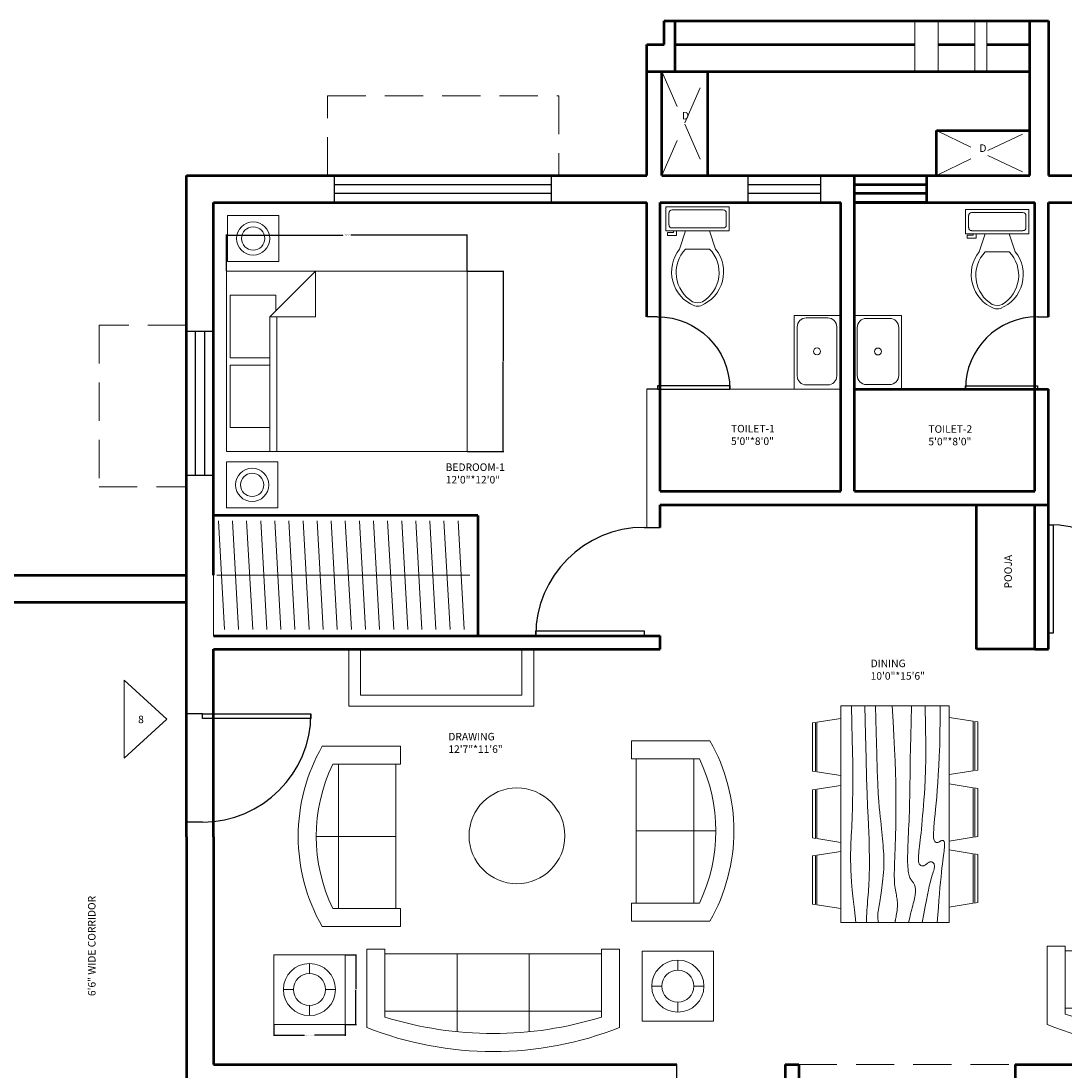
# Model space of a CAD drawing. Units: inches. Extents: x 4795 to 6024, y 2716 to 5025.
# Tile 18 of 19: x 5473 to 5820, y 4676 to 5025. Entities that reach past the tile are written whole.
import ezdxf

# ---------------------------------------------------------------- set-up
doc = ezdxf.new("R2010")
doc.units = ezdxf.units.IN
doc.linetypes.add('DASHED', pattern=[19.05, 12.7, -6.35])
for name, color, linetype, lineweight in [('A-ANNO-DIMS', 2, 'Continuous', 18), ('A-ANNO-TEXT', 7, 'Continuous', 18), ('A-AREA-IDEN', 3, 'Continuous', 18), ('A-DOOR', 4, 'Continuous', 25), ('A-FLOR-FIXT', 9, 'Continuous', 18), ('A-FURN', 8, 'Continuous', 18), ('A-GLAZ', 4, 'Continuous', 25), ('A-WALL', 7, 'Continuous', 50), ('A-WALL-OVHD', 8, 'DASHED', 18)]:
    doc.layers.add(name, color=color, linetype=linetype, lineweight=lineweight)
doc.styles.get("Standard").update_dxf_attribs({"font": 'arial.ttf'})
doc.dimstyles.get("Standard").update_dxf_attribs({"dimtxt": 0.18, "dimasz": 0.18, "dimexe": 0.18, "dimexo": 0.0625, "dimgap": 0.09, "dimtad": 0, "dimtih": 1, "dimtoh": 1, "dimdec": 4, "dimzin": 0, "dimdsep": 46, "dimtxsty": 'Standard', "dimcen": 0.09, "dimadec": 0, "dimazin": 0, "dimtfac": 1, "dimtdec": 4, "dimtofl": 0, "dimtmove": 0, "dimatfit": 3, "dimfxl": 1, "dimtolj": 1, "dimtzin": 0, "dimarcsym": 0})

# ---------------------------------------------------------------- blocks, each defined once
blk = doc.blocks.new('*U2')
for p, q in [((0, 0), (0, -6)), ((40, 0), (40, -6))]:
    blk.add_line(p, q)
blk.add_lwpolyline([(0, 0), (0, 40), (1.75, 40), (1.75, 0)], close=True)
blk.add_arc((0, 0), 40, 0, 90)
blk = doc.blocks.new('Bed - Queen')
for p, q in [((0, -80.00003), (0, 0)), ((0, 0), (59.99999, 0)), ((59.99999, 0), (59.99999, -80.00003)), ((7.99999, -1.2), (28.79998, -1.2)), ((7.99999, -14.4), (7.99999, -1.2)), ((28.79998, -1.2), (28.79998, -14.4)), ((31.19999, -1.2), (51.99999, -1.2)), ((31.19999, -14.4), (31.19999, -1.2)), ((51.99999, -1.2), (51.99999, -16.4)), ((0, -14.4), (44.8, -14.4)), ((44.8, -16.8), (0, -16.8)), ((59.99999, -29.6), (44.8, -14.4)), ((44.8, -14.4), (44.8, -29.6)), ((51.99999, -16.4), (46.79936, -16.4)), ((44.8, -29.6), (59.99999, -29.6)), ((59.99999, -80.00003), (0, -80.00003))]:
    blk.add_line(p, q)
blk = doc.blocks.new('Toilet - top')
for p, q in [((9.5, -6), (9.5, -2)), ((-10, -8.5), (-8, -8.5)), ((-10, -9.5), (-10, -8.5)), ((-7, -9.5), (-10, -9.5)), ((-8, -8.5), (-8, -8)), ((-7, -8), (-7, -9.5)), ((-4, -8), (-6, -14)), ((4, -8), (6, -14)), ((4, -14), (-4, -14))]:
    blk.add_line(p, q)
blk.add_lwpolyline([(10.5, -8), (10.5, 0), (-10.5, 0), (-10.5, -8)], close=True)
for points in [[(-9.5, -2), (-9.5, -6)], [(8.5, -1), (-8.5, -1)], [(-8.5, -7), (8.5, -7)]]:
    blk.add_lwpolyline(points)
for centre, radius, start, end in [((-8.62, -1.88), 0.884, 81.8699, 188.1301), ((8.62, -1.88), 0.884, 351.8699, 98.1301), ((-8.62, -6.12), 0.884, 171.8699, 278.1301), ((8.62, -6.12), 0.884, 261.8699, 8.1301), ((3.52, -21.58), 12.17, 141.4691, 247.9714), ((4.2, -21.82), 11.33, 136.3677, 238.9468), ((-3.52, -21.58), 12.17, 292.0284, 38.5307), ((-4.2, -21.82), 11.33, 301.053, 43.6321), ((0, -27.88), 4, 245.7318, 294.2682), ((0, -29), 4, 254.8605, 285.1395)]:
    blk.add_arc(centre, radius, start, end)
blk = doc.blocks.new('Sofa - Roundback 7 ft.')
for p, q in [((-12.00002, -32.4421), (-12.00003, -6.5971)), ((11.99997, -32.4421), (11.99998, -6.5971)), ((-36.000027, -34), (-36.000027, -11.4696)), ((-35.999844, -13.3819), (35.9998, -13.3819)), ((35.99998, -34), (35.99998, -11.4696)), ((-36.000027, -32.4421), (35.99998, -32.4421))]:
    blk.add_line(p, q)
for points in [[(-36.000027, -34), (-42.000027, -34), (-42.000027, -8)], [(41.99998, -8), (41.99998, -34), (35.99998, -34)]]:
    blk.add_lwpolyline(points)
for centre, radius, start, end in [((0, -114.25), 114.25, 68.43141, 111.5686), ((-0.00001, -127.1968), 121.1968, 72.72033, 107.2797)]:
    blk.add_arc(centre, radius, start, end)
blk = doc.blocks.new('Sofa - Roundback Loveseat 5 ft.')
for p, q in [((0, -32.44198), (0, -5.99998)), ((-24, -33.99998), (-24, -11.46958)), ((-23.9998, -13.38178), (23.99986, -13.38178)), ((24.00004, -33.99998), (24.00004, -11.46958)), ((-24, -32.44198), (24.00004, -32.44198))]:
    blk.add_line(p, q)
for points in [[(-24, -33.99998), (-30, -33.99998), (-30, -7.99998)], [(30.00004, -7.99998), (30.00004, -33.99998), (24.00004, -33.99998)]]:
    blk.add_lwpolyline(points)
for centre, radius, start, end in [((0, -60.24998), 60.24998, 60.13715, 119.8628), ((0, -61.38438), 55.38444, 64.32083, 115.6792)]:
    blk.add_arc(centre, radius, start, end)
blk = doc.blocks.new('WIN-48')
for p, q in [((0, 0), (0, 48)), ((0, 48), (9, 48)), ((3, 0), (3, 48)), ((6, 48), (6, 0)), ((9, 48), (9, 0)), ((9, 0), (0, 0))]:
    blk.add_line(p, q)
blk = doc.blocks.new('WIN-72')
for p, q in [((0, 0), (0, 9)), ((0, 9), (72, 9)), ((72, 9), (72, 0)), ((0, 6), (72, 6)), ((72, 3), (0, 3)), ((72, 0), (0, 0))]:
    blk.add_line(p, q)
blk = doc.blocks.new('WIN-24')
for p, q in [((0, 0), (0, 9)), ((0, 9), (24, 9)), ((24, 9), (24, 0)), ((0, 6), (24, 6)), ((24, 3), (0, 3)), ((24, 0), (0, 0))]:
    blk.add_line(p, q)
blk = doc.blocks.new('CHAIR-DINING')
for p, q in [((8, 17.72), (0, 18.97)), ((8, 17.71), (8, 1.25)), ((9.5, 17.48), (8.5, 17.64)), ((8.5, 1.33), (8.5, 17.64)), ((9.5, 17.48), (9.5, 1.48)), ((0, 0), (8, 1.25)), ((8.5, 1.33), (9.5, 1.48))]:
    blk.add_line(p, q)
blk = doc.blocks.new('LAMP-SIDE')
for p, q in [((11.88, 20.25), (11.88, 16.92)), ((3.23, 11.6), (6.56, 11.6)), ((17.2, 11.6), (20.54, 11.6)), ((11.88, 6.28), (11.88, 2.94))]:
    blk.add_line(p, q)
blk.add_lwpolyline([(23.76, 23.19), (0, 23.19), (0, 0), (23.76, 0)], close=True)
for radius in [8.66, 5.32]:
    blk.add_circle((11.88, 11.6), radius)
blk = doc.blocks.new('*D23')
at = {"layer": 'A-ANNO-DIMS', "color": 0, "lineweight": -2, "transparency": 16777216}
for p, q in [((5557.24, 4691.68), (5557.24, 4688)), ((5581, 4691.68), (5581, 4688)), ((5557.42, 4688.18), (5567.46, 4688.18)), ((5580.82, 4688.18), (5570.79, 4688.18))]:
    blk.add_line(p, q, dxfattribs=at)
at = {"layer": 'A-ANNO-DIMS', "color": 0, "lineweight": 100, "transparency": 16777216}
for points in [[(5557.42, 4688.21), (5557.42, 4688.15), (5557.24, 4688.18)], [(5580.82, 4688.21), (5580.82, 4688.15), (5581, 4688.18)]]:
    blk.add_solid(points, dxfattribs=at)
at = {"layer": 'DEFPOINTS', "color": 0, "lineweight": 100, "transparency": 16777216}
for p in [(5557.24, 4691.74), (5581, 4691.74), (5581, 4688.18)]:
    blk.add_point(p, dxfattribs=at)
at = {"layer": 'A-ANNO-DIMS', "color": 0, "transparency": 16777216, "insert": (5569.12, 4688.18), "char_height": 0.18, "attachment_point": 5}
blk.add_mtext('\\A1;SIDE TABLE LAMP 24 TYP.', dxfattribs=at)
blk = doc.blocks.new('*D24')
at = {"layer": 'A-ANNO-DIMS', "color": 0, "lineweight": -2, "transparency": 16777216}
for p, q in [((5581.07, 4714.94), (5584.75, 4714.94)), ((5584.57, 4714.76), (5584.57, 4703.52)), ((5584.57, 4691.92), (5584.57, 4703.16)), ((5581.07, 4691.74), (5584.75, 4691.74))]:
    blk.add_line(p, q, dxfattribs=at)
at = {"layer": 'A-ANNO-DIMS', "color": 0, "lineweight": 100, "transparency": 16777216}
for points in [[(5584.54, 4714.76), (5584.6, 4714.76), (5584.57, 4714.94)], [(5584.54, 4691.92), (5584.6, 4691.92), (5584.57, 4691.74)]]:
    blk.add_solid(points, dxfattribs=at)
at = {"layer": 'DEFPOINTS', "color": 0, "lineweight": 100, "transparency": 16777216}
for p in [(5581, 4714.94), (5584.57, 4714.94), (5581, 4691.74)]:
    blk.add_point(p, dxfattribs=at)
at = {"layer": 'A-ANNO-DIMS', "color": 0, "transparency": 16777216, "insert": (5584.57, 4703.34), "char_height": 0.18, "attachment_point": 5}
blk.add_mtext('\\A1;23 TYP.', dxfattribs=at)
blk = doc.blocks.new('*D25')
at = {"layer": 'A-ANNO-DIMS', "color": 0, "lineweight": -2, "transparency": 16777216}
for p, q in [((5541.53, 4942.23), (5541.53, 4954.35)), ((5541.71, 4954.17), (5580.22, 4954.17)), ((5621.35, 4954.17), (5582.83, 4954.17)), ((5621.53, 4942.23), (5621.53, 4954.35))]:
    blk.add_line(p, q, dxfattribs=at)
at = {"layer": 'A-ANNO-DIMS', "color": 0, "lineweight": 100, "transparency": 16777216}
for points in [[(5541.71, 4954.2), (5541.71, 4954.14), (5541.53, 4954.17)], [(5621.35, 4954.2), (5621.35, 4954.14), (5621.53, 4954.17)]]:
    blk.add_solid(points, dxfattribs=at)
at = {"layer": 'DEFPOINTS', "color": 0, "lineweight": 100, "transparency": 16777216}
for p in [(5541.53, 4954.17), (5541.53, 4942.17), (5621.53, 4942.17)]:
    blk.add_point(p, dxfattribs=at)
at = {"layer": 'A-ANNO-DIMS', "color": 0, "transparency": 16777216, "insert": (5581.53, 4954.17), "char_height": 0.18, "attachment_point": 5}
blk.add_mtext('\\A1;QUEEN BED 80 TYP.', dxfattribs=at)
blk = doc.blocks.new('*D26')
at = {"layer": 'A-ANNO-DIMS', "color": 0, "lineweight": -2, "transparency": 16777216}
for p, q in [((5621.59, 4942.17), (5633.71, 4942.17)), ((5633.53, 4941.99), (5633.53, 4912.35)), ((5633.53, 4882.35), (5633.53, 4911.99)), ((5621.59, 4882.17), (5633.71, 4882.17))]:
    blk.add_line(p, q, dxfattribs=at)
at = {"layer": 'A-ANNO-DIMS', "color": 0, "lineweight": 100, "transparency": 16777216}
for points in [[(5633.5, 4941.99), (5633.56, 4941.99), (5633.53, 4942.17)], [(5633.5, 4882.35), (5633.56, 4882.35), (5633.53, 4882.17)]]:
    blk.add_solid(points, dxfattribs=at)
at = {"layer": 'DEFPOINTS', "color": 0, "lineweight": 100, "transparency": 16777216}
for p in [(5621.53, 4942.17), (5633.53, 4942.17), (5621.53, 4882.17)]:
    blk.add_point(p, dxfattribs=at)
at = {"layer": 'A-ANNO-DIMS', "color": 0, "transparency": 16777216, "insert": (5633.53, 4912.17), "char_height": 0.18, "attachment_point": 5}
blk.add_mtext('\\A1;60 TYP.', dxfattribs=at)

msp = doc.modelspace()

# ---------------------------------------------------------------- linework, layer by layer
at = {"layer": 'A-FLOR-FIXT'}
for points in [[(5745.72, 4902.99), (5730.23, 4902.99), (5730.23, 4927.41), (5745.72, 4927.41)], [(5750.22, 4902.99), (5765.94, 4902.99), (5765.94, 4927.41), (5750.22, 4927.41)]]:
    msp.add_lwpolyline(points, close=True, dxfattribs=at)
for points in [[(5734.23, 4926.65), (5741.38, 4926.65, -0.414214), (5744.38, 4923.65), (5744.38, 4907.34, -0.414214), (5741.38, 4904.34), (5734.23, 4904.34, -0.414214), (5731.23, 4907.34), (5731.23, 4923.65, -0.414214)], [(5754.16, 4926.44), (5761.96, 4926.44, -0.414214), (5764.96, 4923.44), (5764.96, 4907.49, -0.414214), (5761.96, 4904.49), (5754.16, 4904.49, -0.414214), (5751.16, 4907.49), (5751.16, 4923.44, -0.414214)]]:
    msp.add_lwpolyline(points, format="xyb", close=True, dxfattribs=at)
for centre in [(5737.81, 4915.49), (5758.06, 4915.47)]:
    msp.add_circle(centre, 1.15, dxfattribs=at)
at = {"layer": 'A-FURN'}
for p, q in [((5681.22, 4902.99), (5745.72, 4902.99)), ((5681.22, 4856.98), (5681.22, 4902.99)), ((5538.87, 4859.18), (5540.89, 4823.01)), ((5543.56, 4859.18), (5545.57, 4823.01)), ((5548.24, 4859.18), (5550.26, 4823.01)), ((5552.93, 4859.18), (5554.95, 4823.01)), ((5557.61, 4859.18), (5559.63, 4823.01)), ((5562.3, 4859.18), (5564.32, 4823.01)), ((5566.98, 4859.18), (5569, 4823.01)), ((5571.67, 4859.18), (5573.69, 4823.01)), ((5576.36, 4859.18), (5578.37, 4823.01)), ((5581.04, 4859.18), (5583.06, 4823.01)), ((5585.73, 4859.18), (5587.75, 4823.01)), ((5590.41, 4859.18), (5592.43, 4823.01)), ((5595.1, 4859.18), (5597.12, 4823.01)), ((5599.78, 4859.18), (5601.8, 4823.01)), ((5604.47, 4859.18), (5606.49, 4823.01)), ((5609.16, 4859.18), (5611.17, 4823.01)), ((5613.84, 4859.18), (5615.86, 4823.01)), ((5618.53, 4859.18), (5620.55, 4823.01)), ((5537.22, 4820.98), (5537.22, 4841.09)), ((5538.32, 4841.1), (5622.4, 4841.1)), ((5582.22, 4816.48), (5582.22, 4797.51)), ((5586.13, 4816.48), (5586.13, 4801.2)), ((5639.68, 4801.2), (5639.68, 4816.48)), ((5643.75, 4797.51), (5643.75, 4816.48)), ((5507.59, 4806.23), (5507.59, 4780.26)), ((5521.76, 4793.24), (5507.59, 4806.23)), ((5586.13, 4801.2), (5639.68, 4801.2)), ((5582.22, 4797.51), (5643.75, 4797.51)), ((5745.76, 4797.66), (5745.76, 4725.66)), ((5781.76, 4797.66), (5745.76, 4797.66)), ((5781.76, 4725.66), (5781.76, 4797.66)), ((5507.59, 4780.26), (5521.76, 4793.24)), ((5745.76, 4725.66), (5781.76, 4725.66))]:
    msp.add_line(p, q, dxfattribs=at)
for points in [[(5770.32, 5025.34), (5778.07, 5025.34), (5778.07, 5008.52), (5770.32, 5008.52)], [(5790.29, 5025.34), (5794.24, 5025.34), (5794.24, 5008.52), (5790.29, 5008.52)], [(5541.86, 4960.71), (5558.98, 4960.71), (5558.98, 4945.37), (5541.86, 4945.37)], [(5541.53, 4878.78), (5558.65, 4878.78), (5558.65, 4863.44), (5541.53, 4863.44)]]:
    msp.add_lwpolyline(points, close=True, dxfattribs=at)
for points in [[(5749.26, 4797.66), (5749.43, 4791.75), (5749.55, 4786.69), (5749.64, 4782.39), (5749.69, 4778.74), (5749.72, 4775.63), (5749.72, 4772.96), (5749.71, 4770.63), (5749.68, 4768.53), (5749.65, 4766.58), (5749.6, 4764.75), (5749.56, 4763.03), (5749.5, 4761.41), (5749.45, 4759.89), (5749.39, 4758.46), (5749.33, 4757.11), (5749.26, 4755.83), (5749.2, 4754.6), (5749.14, 4753.42), (5749.09, 4752.27), (5749.04, 4751.11), (5749, 4749.94), (5748.98, 4748.73), (5748.97, 4747.46), (5748.97, 4746.12), (5749, 4744.67), (5749.06, 4743.04), (5749.16, 4741.18), (5749.32, 4739), (5749.55, 4736.43), (5749.86, 4733.4), (5750.26, 4729.83), (5750.76, 4725.66)], [(5753.76, 4797.66), (5753.95, 4788.06), (5754.13, 4780.13), (5754.31, 4773.64), (5754.48, 4768.4), (5754.64, 4764.18), (5754.78, 4760.78), (5754.91, 4757.98), (5755.01, 4755.58), (5755.1, 4753.38), (5755.16, 4751.36), (5755.2, 4749.49), (5755.22, 4747.76), (5755.23, 4746.17), (5755.22, 4744.7), (5755.21, 4743.34), (5755.18, 4742.08), (5755.15, 4740.9), (5755.1, 4739.79), (5755.05, 4738.74), (5755, 4737.73), (5754.94, 4736.75), (5754.87, 4735.78), (5754.8, 4734.81), (5754.72, 4733.83), (5754.64, 4732.81), (5754.56, 4731.78), (5754.49, 4730.73), (5754.41, 4729.68), (5754.35, 4728.64), (5754.31, 4727.61), (5754.27, 4726.62), (5754.26, 4725.66)], [(5757.26, 4797.66), (5757.45, 4788.84), (5757.64, 4781.74), (5757.82, 4776.13), (5758, 4771.77), (5758.18, 4768.43), (5758.35, 4765.9), (5758.52, 4763.92), (5758.68, 4762.28), (5758.83, 4760.79), (5758.98, 4759.39), (5759.11, 4758.07), (5759.24, 4756.83), (5759.36, 4755.65), (5759.48, 4754.53), (5759.58, 4753.45), (5759.68, 4752.41), (5759.77, 4751.39), (5759.85, 4750.39), (5759.92, 4749.39), (5759.97, 4748.41), (5760.01, 4747.42), (5760.03, 4746.43), (5760.03, 4745.43), (5760.01, 4744.41), (5759.97, 4743.37), (5759.91, 4742.31), (5759.83, 4741.26), (5759.73, 4740.21), (5759.63, 4739.18), (5759.51, 4738.19), (5759.39, 4737.23), (5759.26, 4736.33), (5759.14, 4735.48), (5759.01, 4734.69), (5758.89, 4733.94), (5758.77, 4733.24), (5758.65, 4732.56), (5758.53, 4731.9), (5758.42, 4731.26), (5758.31, 4730.62), (5758.2, 4729.98), (5758.11, 4729.33), (5758.03, 4728.69), (5757.99, 4728.06), (5757.98, 4727.44), (5758.02, 4726.83), (5758.11, 4726.23), (5758.26, 4725.66)], [(5762.76, 4797.66), (5763.1, 4792.45), (5763.38, 4787.68), (5763.6, 4783.31), (5763.77, 4779.32), (5763.89, 4775.66), (5763.98, 4772.31), (5764.03, 4769.24), (5764.06, 4766.41), (5764.06, 4763.79), (5764.05, 4761.37), (5764.03, 4759.13), (5763.99, 4757.04), (5763.94, 4755.11), (5763.89, 4753.3), (5763.83, 4751.6), (5763.76, 4749.99), (5763.7, 4748.47), (5763.64, 4747.02), (5763.59, 4745.66), (5763.55, 4744.38), (5763.51, 4743.18), (5763.49, 4742.06), (5763.49, 4741.02), (5763.51, 4740.08), (5763.56, 4739.21), (5763.62, 4738.42), (5763.7, 4737.7), (5763.78, 4737.04), (5763.88, 4736.44), (5763.98, 4735.87), (5764.08, 4735.33), (5764.18, 4734.83), (5764.27, 4734.33), (5764.35, 4733.85), (5764.42, 4733.37), (5764.47, 4732.89), (5764.51, 4732.4), (5764.53, 4731.9), (5764.53, 4731.37), (5764.51, 4730.83), (5764.47, 4730.25), (5764.41, 4729.66), (5764.34, 4729.07), (5764.25, 4728.5), (5764.17, 4727.96), (5764.08, 4727.47), (5764, 4727.04), (5763.93, 4726.7), (5763.88, 4726.45), (5763.83, 4726.27), (5763.8, 4726.16), (5763.78, 4726.07), (5763.77, 4726), (5763.77, 4725.92), (5763.76, 4725.81), (5763.76, 4725.66)], [(5769.26, 4797.66), (5769.1, 4792.37), (5768.97, 4787.73), (5768.88, 4783.65), (5768.82, 4780.09), (5768.77, 4776.96), (5768.74, 4774.21), (5768.71, 4771.77), (5768.68, 4769.58), (5768.65, 4767.57), (5768.6, 4765.72), (5768.56, 4764), (5768.5, 4762.4), (5768.45, 4760.89), (5768.39, 4759.44), (5768.33, 4758.04), (5768.26, 4756.66), (5768.2, 4755.29), (5768.14, 4753.92), (5768.09, 4752.59), (5768.03, 4751.28), (5767.99, 4750.03), (5767.96, 4748.83), (5767.94, 4747.7), (5767.93, 4746.66), (5767.94, 4745.71), (5767.96, 4744.84), (5768, 4744.06), (5768.06, 4743.36), (5768.13, 4742.73), (5768.21, 4742.17), (5768.31, 4741.68), (5768.43, 4741.24), (5768.56, 4740.86), (5768.71, 4740.53), (5768.86, 4740.23), (5769.02, 4739.97), (5769.19, 4739.73), (5769.36, 4739.51), (5769.52, 4739.29), (5769.68, 4739.08), (5769.83, 4738.85), (5769.97, 4738.62), (5770.11, 4738.37), (5770.22, 4738.11), (5770.32, 4737.82), (5770.41, 4737.52), (5770.47, 4737.19), (5770.51, 4736.83), (5770.53, 4736.44), (5770.53, 4736.02), (5770.51, 4735.57), (5770.46, 4735.11), (5770.4, 4734.62), (5770.31, 4734.12), (5770.21, 4733.6), (5770.1, 4733.08), (5769.96, 4732.53), (5769.81, 4731.95), (5769.63, 4731.29), (5769.43, 4730.52), (5769.2, 4729.61), (5768.93, 4728.52), (5768.62, 4727.21), (5768.26, 4725.66)], [(5773.76, 4797.66), (5773.91, 4790.64), (5773.97, 4784.83), (5773.96, 4780.08), (5773.9, 4776.23), (5773.79, 4773.1), (5773.66, 4770.54), (5773.51, 4768.37), (5773.35, 4766.45), (5773.19, 4764.63), (5773.05, 4762.88), (5772.91, 4761.22), (5772.77, 4759.63), (5772.64, 4758.13), (5772.52, 4756.72), (5772.39, 4755.39), (5772.26, 4754.16), (5772.14, 4753.02), (5772.02, 4751.97), (5771.9, 4751.01), (5771.8, 4750.13), (5771.7, 4749.33), (5771.62, 4748.62), (5771.56, 4747.98), (5771.51, 4747.41), (5771.49, 4746.91), (5771.5, 4746.48), (5771.52, 4746.11), (5771.57, 4745.78), (5771.63, 4745.51), (5771.71, 4745.28), (5771.81, 4745.08), (5771.93, 4744.91), (5772.06, 4744.76), (5772.21, 4744.64), (5772.37, 4744.55), (5772.53, 4744.48), (5772.71, 4744.44), (5772.89, 4744.43), (5773.08, 4744.45), (5773.26, 4744.49), (5773.45, 4744.57), (5773.64, 4744.67), (5773.83, 4744.79), (5774.01, 4744.93), (5774.2, 4745.07), (5774.39, 4745.22), (5774.58, 4745.36), (5774.76, 4745.49), (5774.95, 4745.61), (5775.14, 4745.71), (5775.32, 4745.78), (5775.5, 4745.84), (5775.68, 4745.86), (5775.85, 4745.86), (5776.02, 4745.82), (5776.18, 4745.74), (5776.33, 4745.63), (5776.47, 4745.48), (5776.6, 4745.3), (5776.7, 4745.09), (5776.78, 4744.85), (5776.84, 4744.58), (5776.86, 4744.3), (5776.85, 4743.99), (5776.8, 4743.67), (5776.71, 4743.32), (5776.59, 4742.92), (5776.45, 4742.47), (5776.27, 4741.94), (5776.08, 4741.33), (5775.87, 4740.61), (5775.64, 4739.78), (5775.4, 4738.82), (5775.14, 4737.7), (5774.85, 4736.38), (5774.53, 4734.83), (5774.17, 4733.02), (5773.76, 4730.91), (5773.29, 4728.47), (5772.76, 4725.66)], [(5778.76, 4797.66), (5778.74, 4792.84), (5778.68, 4788.47), (5778.58, 4784.51), (5778.45, 4780.94), (5778.3, 4777.7), (5778.13, 4774.75), (5777.95, 4772.07), (5777.76, 4769.62), (5777.58, 4767.35), (5777.39, 4765.26), (5777.22, 4763.35), (5777.06, 4761.62), (5776.91, 4760.06), (5776.78, 4758.68), (5776.67, 4757.46), (5776.6, 4756.41), (5776.55, 4755.52), (5776.53, 4754.78), (5776.54, 4754.17), (5776.58, 4753.68), (5776.63, 4753.29), (5776.71, 4752.99), (5776.81, 4752.75), (5776.93, 4752.58), (5777.06, 4752.44), (5777.21, 4752.34), (5777.36, 4752.27), (5777.52, 4752.23), (5777.69, 4752.22), (5777.86, 4752.24), (5778.02, 4752.27), (5778.18, 4752.33), (5778.33, 4752.4), (5778.48, 4752.48), (5778.62, 4752.56), (5778.75, 4752.65), (5778.88, 4752.73), (5779.01, 4752.81), (5779.14, 4752.87), (5779.26, 4752.91), (5779.39, 4752.93), (5779.51, 4752.92), (5779.63, 4752.9), (5779.74, 4752.85), (5779.85, 4752.77), (5779.94, 4752.67), (5780.03, 4752.55), (5780.1, 4752.41), (5780.15, 4752.24), (5780.19, 4752.04), (5780.21, 4751.81), (5780.22, 4751.53), (5780.21, 4751.21), (5780.19, 4750.84), (5780.15, 4750.41), (5780.1, 4749.91), (5780.03, 4749.34), (5779.94, 4748.69), (5779.84, 4747.94), (5779.73, 4747.09), (5779.61, 4746.12), (5779.48, 4745.02), (5779.33, 4743.77), (5779.18, 4742.37), (5779.02, 4740.8), (5778.85, 4739.07), (5778.68, 4737.19), (5778.5, 4735.15), (5778.32, 4732.98), (5778.14, 4730.67), (5777.95, 4728.22), (5777.76, 4725.66)]]:
    msp.add_lwpolyline(points, dxfattribs=at)
for centre, radius in [((5550.42, 4953.04), 5.52), ((5550.42, 4953.04), 3.86), ((5550.09, 4871.11), 5.52), ((5550.09, 4871.11), 3.86), ((5638.08, 4754.47), 15.92)]:
    msp.add_circle(centre, radius, dxfattribs=at)
at = {"layer": 'A-WALL'}
for p, q in [((5686.98, 5017.52), (5686.98, 5025.34)), ((5686.98, 5025.34), (5690.61, 5025.34)), ((5690.61, 5025.34), (5690.61, 5008.52)), ((5690.61, 5025.34), (5814.72, 5025.34)), ((5808.49, 4973.98), (5808.49, 5025.34)), ((5814.72, 5025.34), (5814.72, 5025.34)), ((5814.72, 5025.34), (5814.72, 5017.52)), ((5681.22, 4973.98), (5681.22, 5017.52)), ((5681.22, 5017.52), (5686.98, 5017.52)), ((5690.61, 5017.52), (5770.32, 5017.52)), ((5778.07, 5017.52), (5790.29, 5017.52)), ((5794.24, 5017.52), (5808.49, 5017.52)), ((5814.72, 5017.52), (5814.72, 4973.98)), ((5681.22, 5008.52), (5808.49, 5008.52)), ((5686.29, 4973.98), (5686.29, 5008.52)), ((5701.37, 5008.52), (5701.37, 4973.98)), ((5777.48, 4973.98), (5777.48, 4988.93)), ((5777.48, 4988.93), (5808.49, 4988.93)), ((5528.22, 4841.09), (5528.22, 4973.98)), ((5528.22, 4973.98), (5681.22, 4973.98)), ((5686.29, 4973.98), (5808.49, 4973.98)), ((5750.22, 4868.98), (5750.22, 4973.98)), ((5750.22, 4973.98), (5774.22, 4973.98)), ((5750.22, 4964.98), (5750.22, 4973.98)), ((5750.22, 4970.98), (5774.22, 4970.98)), ((5774.22, 4973.98), (5774.22, 4964.98)), ((5814.72, 4973.98), (5955.72, 4973.98)), ((5774.22, 4967.98), (5750.22, 4967.98)), ((5537.22, 4841.09), (5537.22, 4964.98)), ((5537.22, 4964.98), (5681.22, 4964.98)), ((5681.22, 4926.99), (5681.22, 4964.98)), ((5685.72, 4964.98), (5745.72, 4964.98)), ((5685.72, 4868.98), (5685.72, 4964.98)), ((5745.72, 4868.98), (5745.72, 4964.98)), ((5774.22, 4964.98), (5750.22, 4964.98)), ((5750.22, 4964.98), (5810.22, 4964.98)), ((5810.22, 4868.98), (5810.22, 4964.98)), ((5814.72, 4964.98), (5946.72, 4964.98)), ((5814.72, 4926.99), (5814.72, 4964.98)), ((5750.22, 4902.99), (5814.72, 4902.99)), ((5814.72, 4816.48), (5814.72, 4902.99)), ((5685.72, 4868.98), (5745.72, 4868.98)), ((5750.22, 4868.98), (5810.22, 4868.98)), ((5685.72, 4864.48), (5814.72, 4864.48)), ((5685.72, 4856.98), (5685.72, 4864.48)), ((5790.84, 4816.48), (5790.84, 4864.48)), ((5810.22, 4816.48), (5810.22, 4864.48)), ((5625.11, 4860.89), (5537.22, 4860.89)), ((5625.11, 4860.89), (5625.11, 4820.98)), ((5286.97, 4841.09), (5528.22, 4841.09)), ((5528.22, 4754.09), (5528.22, 4841.09)), ((5286.97, 4832.09), (5528.22, 4832.09)), ((5537.22, 4820.98), (5685.72, 4820.98)), ((5685.72, 4816.48), (5685.72, 4820.98)), ((5537.22, 4754.09), (5537.22, 4816.48)), ((5537.22, 4816.48), (5685.72, 4816.48)), ((5810.22, 4816.48), (5790.84, 4816.48)), ((5810.22, 4816.48), (5814.72, 4816.48)), ((5528.22, 4754.09), (5528.22, 4616.09)), ((5537.22, 4754.09), (5537.22, 4678.48)), ((5537.22, 4678.48), (5691.22, 4678.48)), ((5727.22, 4678.48), (5727.22, 4582.12)), ((5727.22, 4678.48), (5731.72, 4678.48)), ((5731.72, 4678.48), (5731.72, 4629.48)), ((5803.72, 4678.48), (5803.72, 4673.98)), ((5803.72, 4678.48), (5955.72, 4678.48))]:
    msp.add_line(p, q, dxfattribs=at)
at = {"layer": 'A-WALL-OVHD'}
for p, q in [((5686.29, 5008.52), (5701.37, 4973.98)), ((5686.29, 4973.98), (5701.37, 5008.52)), ((5701.37, 5008.52), (5701.37, 5008.52)), ((5575.14, 4973.98), (5575.14, 5000.44)), ((5575.14, 5000.44), (5652.05, 5000.44)), ((5652.05, 5000.44), (5652.05, 4973.98)), ((5777.48, 4988.93), (5808.49, 4973.98)), ((5777.48, 4973.98), (5808.49, 4988.93)), ((5528.12, 4924.19), (5499.21, 4924.19)), ((5499.21, 4924.19), (5499.21, 4870.5)), ((5499.21, 4870.5), (5528.22, 4870.5)), ((5731.72, 4678.48), (5803.72, 4678.48))]:
    msp.add_line(p, q, dxfattribs=at)

# ---------------------------------------------------------------- block references
at = {"layer": 'A-DOOR'}
for p, xscale, yscale, zscale, rotation in [((5684.82, 4902.99), -0.6, 0.6, 0.6, 270), ((5811.12, 4902.99), 0.6, 0.6, 0.6, 90.00000000000003), ((5680.32, 4820.98), 0.9, 0.9, 0.9, 90), ((5533.62, 4795.04), 0.9, 0.9, 0.9, 270), ((5727.22, 4673.08), 0.9, 0.9, 0.9, 180)]:
    msp.add_blockref('*U2', p, dxfattribs=dict(at, xscale=xscale, yscale=yscale, zscale=zscale, rotation=rotation))
at = {"layer": 'A-DOOR', "xscale": 0.9, "yscale": 0.9, "zscale": 0.9}
msp.add_blockref('*U2', (5814.72, 4821.88), dxfattribs=at)
at = {"layer": 'A-FLOR-FIXT'}
for p in [(5698.12, 4963.53), (5797.71, 4962.63)]:
    msp.add_blockref('Toilet - top', p, dxfattribs=at)
at = {"layer": 'A-FURN'}
for name, p, rotation in [('Bed - Queen', (5541.53, 4882.17), 90), ('CHAIR-DINING', (5745.76, 4793.46), 180.0056718243519), ('Sofa - Roundback Loveseat 5 ft.', (5710.2, 4756.06), 270), ('Sofa - Roundback Loveseat 5 ft.', (5565.39, 4754.26), 90), ('CHAIR-DINING', (5745.76, 4771.24), 180.0056718243519), ('CHAIR-DINING', (5745.76, 4749.26), 180.0056718243519), ('Sofa - Roundback 7 ft.', (5630.19, 4682.74), 180), ('Sofa - Roundback 7 ft.', (5856.28, 4683.73), 180)]:
    msp.add_blockref(name, p, dxfattribs=dict(at, rotation=rotation))
for name, p in [('CHAIR-DINING', (5781.76, 4774.83)), ('CHAIR-DINING', (5781.76, 4752.73)), ('CHAIR-DINING', (5781.76, 4730.79)), ('LAMP-SIDE', (5679.67, 4692.89)), ('LAMP-SIDE', (5557.24, 4691.75))]:
    msp.add_blockref(name, p, dxfattribs=at)
at = {"layer": 'A-GLAZ', "rotation": 180}
for name, p in [('WIN-72', (5649.43, 4973.98)), ('WIN-24', (5738.97, 4973.98))]:
    msp.add_blockref(name, p, dxfattribs=at)
at = {"layer": 'A-GLAZ'}
msp.add_blockref('WIN-48', (5528.22, 4874.19), dxfattribs=at)

# ---------------------------------------------------------------- texts
at = {"layer": 'A-ANNO-TEXT', "char_height": 2.5, "attachment_point": 1}
for s, width, insert in [('D', 1.486, (5692.91, 4995.13)), ('D', 2.3909, (5791.79, 4984.31)), ('8', 6.049, (5512.18, 4794.41))]:
    msp.add_mtext_dynamic_manual_height_columns(s, width=width, gutter_width=12.5, heights=[0], dxfattribs=dict(at, insert=insert))
at = {"layer": 'A-AREA-IDEN', "char_height": 2.5, "attachment_point": 1}
for s, width, insert in [('TOILET-1\\P5\'0"*8\'0"', 44.0763, (5709.22, 4891.07)), ('TOILET-2\\P5\'0"*8\'0"', 33.4033, (5774.83, 4890.94)), ('BEDROOM-1\\P12\'0"*12\'0"', 55.2352, (5614.41, 4878.26)), ('DINING\\P10\'0"*15\'6"', 37.8294, (5755.63, 4813.02)), ('DRAWING\\P12\'7"*11\'6"', 38.7896, (5615.28, 4788.68))]:
    msp.add_mtext_dynamic_manual_height_columns(s, width=width, gutter_width=12.5, heights=[0], dxfattribs=dict(at, insert=insert))
at = {"layer": 'A-AREA-IDEN', "char_height": 2.5, "attachment_point": 1, "rotation": 90}
for s, width, insert in [('POOJA', 13.6296, (5800.08, 4836.7)), ('6\'6" WIDE CORRIDOR', 46.7744, (5495.53, 4701.18))]:
    msp.add_mtext_dynamic_manual_height_columns(s, width=width, gutter_width=12.5, heights=[0], dxfattribs=dict(at, insert=insert))

# ---------------------------------------------------------------- dimensions: what is measured, and where the dimension line sits
at = {"layer": 'A-ANNO-DIMS'}
for base, p1, p2, angle, text, picture, middle in [((5541.53, 4954.17), (5621.53, 4942.17), (5541.53, 4942.17), 180, 'QUEEN BED <> TYP.', '*D25', (5581.53, 4954.17)), ((5633.53, 4942.17), (5621.53, 4882.17), (5621.53, 4942.17), 90, '<> TYP.', '*D26', (5633.53, 4912.17)), ((5584.57, 4714.94), (5581, 4691.74), (5581, 4714.94), 90, '<> TYP.', '*D24', (5584.57, 4703.34))]:
    dim = msp.add_linear_dim(base=base, p1=p1, p2=p2, angle=angle, text=text, dimstyle='Standard', override={"dimdec": 0, "dimlfac": 1, "dimrnd": 0, "dimzin": 0, "dimdsep": 46, "dimlunit": 2}, dxfattribs=at)
    dim.commit()
    dim.dimension.update_dxf_attribs({"geometry": picture, "text_midpoint": middle})
dim = msp.add_linear_dim(base=(5581, 4688.18), p1=(5557.24, 4691.74), p2=(5581, 4691.74), text='SIDE TABLE LAMP <> TYP.', dimstyle='Standard', override={"dimdec": 0, "dimlfac": 1, "dimrnd": 0, "dimzin": 0, "dimdsep": 46, "dimlunit": 2}, dxfattribs=at)
dim.commit()
dim.dimension.update_dxf_attribs({"geometry": '*D23', "text_midpoint": (5569.12, 4688.18)})

doc.saveas('drawing.dxf')
